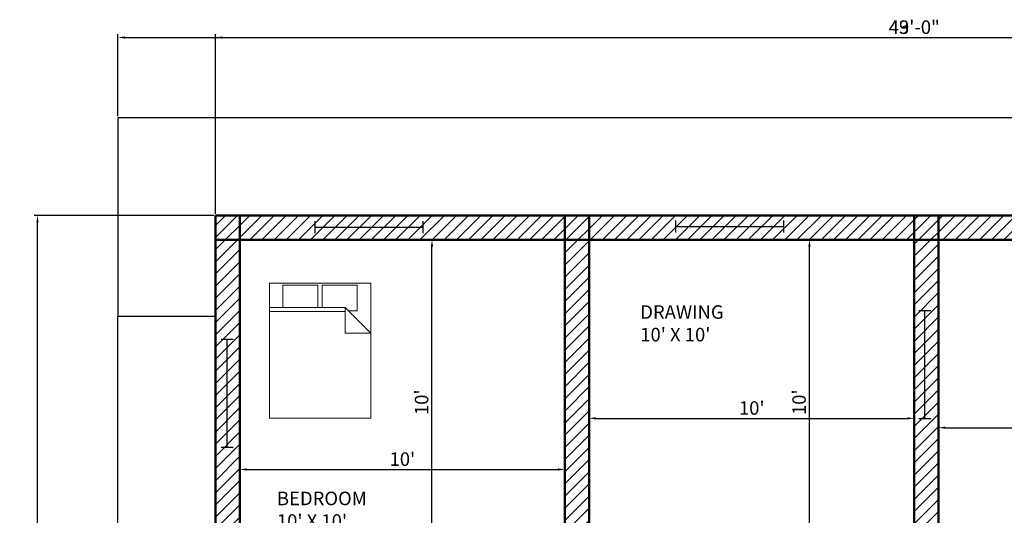
# Model space of a CAD drawing. Units: millimetres. Extents: x 2039 to 2694, y 890 to 1415.
# Tile 3 of 4: x 2039 to 2402, y 1232 to 1415. Entities that reach past the tile are written whole.
import ezdxf

# ---------------------------------------------------------------- set-up
doc = ezdxf.new("R2010")
doc.units = ezdxf.units.MM
for name, color, linetype, lineweight in [('A-ANNO-DIMS', 80, 'Continuous', 18), ('A-AREA-IDEN', 130, 'Continuous', 25), ('A-WALL-PATT', 6, 'Continuous', 13), ('C-PROP', 200, 'Continuous', 25), ('furniture', 140, 'Continuous', 18), ('walls', 200, 'Continuous', 50), ('windows', 30, 'Continuous', 25)]:
    doc.layers.add(name, color=color, linetype=linetype, lineweight=lineweight)
doc.styles.get("Standard").update_dxf_attribs({"font": 'arial.ttf'})
doc.dimstyles.new('ISO-25', dxfattribs={"dimtxt": 5, "dimasz": 2.5, "dimexe": 1.25, "dimexo": 0.625, "dimtad": 1, "dimdec": 0, "dimlunit": 3, "dimtxsty": 'Standard', "dimcen": 2.5, "dimadec": 0, "dimazin": 0, "dimtfac": 1, "dimtdec": 0, "dimtmove": 0, "dimatfit": 3, "dimfxl": 1, "dimarcsym": 0})

# ---------------------------------------------------------------- blocks, each defined once
blk = doc.blocks.new('*U4')
for p, q in [((0, 4), (0, 0)), ((36, 4), (36, 0)), ((0, 2), (36, 2))]:
    blk.add_line(p, q)
blk = doc.blocks.new('Bed - Queen')
for p, q in [((0, -80.00003), (0, 0)), ((0, 0), (59.99999, 0)), ((59.99999, 0), (59.99999, -80.00003)), ((7.99999, -1.2), (28.79998, -1.2)), ((7.99999, -14.4), (7.99999, -1.2)), ((28.79998, -1.2), (28.79998, -14.4)), ((31.19999, -1.2), (51.99999, -1.2)), ((31.19999, -14.4), (31.19999, -1.2)), ((51.99999, -1.2), (51.99999, -16.4)), ((0, -14.4), (44.8, -14.4)), ((44.8, -16.8), (0, -16.8)), ((59.99999, -29.6), (44.8, -14.4)), ((44.8, -14.4), (44.8, -29.6)), ((51.99999, -16.4), (46.79936, -16.4)), ((44.8, -29.6), (59.99999, -29.6)), ((59.99999, -80.00003), (0, -80.00003))]:
    blk.add_line(p, q)
blk = doc.blocks.new('*D8')
at = {"layer": 'A-ANNO-DIMS', "color": 0, "lineweight": -2, "transparency": 16777216}
for p, q in [((2377.91, 1235.18), (2377.91, 1265.13)), ((2617.91, 1235.18), (2617.91, 1265.13)), ((2380.41, 1263.88), (2615.41, 1263.88))]:
    blk.add_line(p, q, dxfattribs=at)
at = {"layer": 'A-ANNO-DIMS', "color": 0, "transparency": 16777216}
for points in [[(2380.41, 1264.3), (2380.41, 1263.46), (2377.91, 1263.88)], [(2615.41, 1264.3), (2615.41, 1263.46), (2617.91, 1263.88)]]:
    blk.add_solid(points, dxfattribs=at)
at = {"layer": 'Defpoints', "color": 0, "transparency": 16777216}
for p in [(2617.91, 1263.88), (2377.91, 1234.56), (2617.91, 1234.56)]:
    blk.add_point(p, dxfattribs=at)
at = {"layer": 'A-ANNO-DIMS', "color": 0, "transparency": 16777216, "insert": (2497.91, 1267.06), "char_height": 5, "attachment_point": 5}
blk.add_mtext("20'", dxfattribs=at)
blk = doc.blocks.new('*D10')
at = {"layer": 'A-ANNO-DIMS', "color": 0, "lineweight": -2, "transparency": 16777216}
for p, q in [((2119.91, 1237.17), (2119.91, 1249.7)), ((2122.41, 1248.45), (2237.41, 1248.45)), ((2239.91, 1237.17), (2239.91, 1249.7))]:
    blk.add_line(p, q, dxfattribs=at)
at = {"layer": 'A-ANNO-DIMS', "color": 0, "transparency": 16777216}
for points in [[(2122.41, 1248.87), (2122.41, 1248.03), (2119.91, 1248.45)], [(2237.41, 1248.87), (2237.41, 1248.03), (2239.91, 1248.45)]]:
    blk.add_solid(points, dxfattribs=at)
at = {"layer": 'Defpoints', "color": 0, "transparency": 16777216}
for p in [(2239.91, 1248.45), (2119.91, 1236.55), (2239.91, 1236.55)]:
    blk.add_point(p, dxfattribs=at)
at = {"layer": 'A-ANNO-DIMS', "color": 0, "transparency": 16777216, "insert": (2179.91, 1251.63), "char_height": 5, "attachment_point": 5}
blk.add_mtext("10'", dxfattribs=at)
blk = doc.blocks.new('*D11')
at = {"layer": 'A-ANNO-DIMS', "color": 0, "lineweight": -2, "transparency": 16777216}
for p, q in [((2187.65, 1333.28), (2192.09, 1333.28)), ((2190.84, 1215.78), (2190.84, 1330.78)), ((2187.65, 1213.28), (2192.09, 1213.28))]:
    blk.add_line(p, q, dxfattribs=at)
at = {"layer": 'A-ANNO-DIMS', "color": 0, "transparency": 16777216}
for points in [[(2190.42, 1330.78), (2191.26, 1330.78), (2190.84, 1333.28)], [(2190.42, 1215.78), (2191.26, 1215.78), (2190.84, 1213.28)]]:
    blk.add_solid(points, dxfattribs=at)
at = {"layer": 'Defpoints', "color": 0, "transparency": 16777216}
for p in [(2187.03, 1333.28), (2190.84, 1333.28), (2187.03, 1213.28)]:
    blk.add_point(p, dxfattribs=at)
at = {"layer": 'A-ANNO-DIMS', "color": 0, "transparency": 16777216, "insert": (2187.66, 1273.28), "char_height": 5, "attachment_point": 5, "rotation": 90}
blk.add_mtext("10'", dxfattribs=at)
blk = doc.blocks.new('*D12')
at = {"layer": 'A-ANNO-DIMS', "color": 0, "lineweight": -2, "transparency": 16777216}
for p, q in [((2248.91, 1295.38), (2248.91, 1266.07)), ((2368.91, 1295.38), (2368.91, 1266.07)), ((2251.41, 1267.32), (2366.41, 1267.32))]:
    blk.add_line(p, q, dxfattribs=at)
at = {"layer": 'A-ANNO-DIMS', "color": 0, "transparency": 16777216}
for points in [[(2251.41, 1267.74), (2251.41, 1266.91), (2248.91, 1267.32)], [(2366.41, 1267.74), (2366.41, 1266.91), (2368.91, 1267.32)]]:
    blk.add_solid(points, dxfattribs=at)
at = {"layer": 'Defpoints', "color": 0, "transparency": 16777216}
for p in [(2248.91, 1296.01), (2368.91, 1296.01), (2368.91, 1267.32)]:
    blk.add_point(p, dxfattribs=at)
at = {"layer": 'A-ANNO-DIMS', "color": 0, "transparency": 16777216, "insert": (2308.91, 1270.5), "char_height": 5, "attachment_point": 5}
blk.add_mtext("10'", dxfattribs=at)
blk = doc.blocks.new('*D13')
at = {"layer": 'A-ANNO-DIMS', "color": 0, "lineweight": -2, "transparency": 16777216}
for p, q in [((2326.26, 1333.28), (2331.46, 1333.28)), ((2330.21, 1215.78), (2330.21, 1330.78)), ((2326.26, 1213.28), (2331.46, 1213.28))]:
    blk.add_line(p, q, dxfattribs=at)
at = {"layer": 'A-ANNO-DIMS', "color": 0, "transparency": 16777216}
for points in [[(2329.79, 1330.78), (2330.63, 1330.78), (2330.21, 1333.28)], [(2329.79, 1215.78), (2330.63, 1215.78), (2330.21, 1213.28)]]:
    blk.add_solid(points, dxfattribs=at)
at = {"layer": 'Defpoints', "color": 0, "transparency": 16777216}
for p in [(2325.64, 1333.28), (2330.21, 1333.28), (2325.64, 1213.28)]:
    blk.add_point(p, dxfattribs=at)
at = {"layer": 'A-ANNO-DIMS', "color": 0, "transparency": 16777216, "insert": (2327.03, 1273.28), "char_height": 5, "attachment_point": 5, "rotation": 90}
blk.add_mtext("10'", dxfattribs=at)
blk = doc.blocks.new('*D35')
at = {"layer": 'A-ANNO-DIMS', "color": 0, "lineweight": -2, "transparency": 16777216}
for p, q in [((2110.91, 1342.9), (2110.91, 1409.23)), ((2113.41, 1407.98), (2624.41, 1407.98)), ((2626.91, 1342.9), (2626.91, 1409.23))]:
    blk.add_line(p, q, dxfattribs=at)
at = {"layer": 'A-ANNO-DIMS', "color": 0, "transparency": 16777216}
for points in [[(2113.41, 1408.39), (2113.41, 1407.56), (2110.91, 1407.98)], [(2624.41, 1408.39), (2624.41, 1407.56), (2626.91, 1407.98)]]:
    blk.add_solid(points, dxfattribs=at)
at = {"layer": 'Defpoints', "color": 0, "transparency": 16777216}
for p in [(2626.91, 1407.98), (2110.91, 1342.28), (2626.91, 1342.28)]:
    blk.add_point(p, dxfattribs=at)
at = {"layer": 'A-ANNO-DIMS', "color": 0, "transparency": 16777216, "insert": (2368.91, 1411.16), "char_height": 5, "attachment_point": 5}
blk.add_mtext('43\'-0"', dxfattribs=at)
blk = doc.blocks.new('*D36')
at = {"layer": 'A-ANNO-DIMS', "color": 0, "lineweight": -2, "transparency": 16777216}
for p, q in [((2110.28, 1342.28), (2043.96, 1342.28)), ((2045.21, 941.78), (2045.21, 1339.78)), ((2110.28, 939.28), (2043.96, 939.28))]:
    blk.add_line(p, q, dxfattribs=at)
at = {"layer": 'A-ANNO-DIMS', "color": 0, "transparency": 16777216}
for points in [[(2044.79, 1339.78), (2045.62, 1339.78), (2045.21, 1342.28)], [(2044.79, 941.78), (2045.62, 941.78), (2045.21, 939.28)]]:
    blk.add_solid(points, dxfattribs=at)
at = {"layer": 'Defpoints', "color": 0, "transparency": 16777216}
for p in [(2045.21, 1342.28), (2110.91, 1342.28), (2110.91, 939.28)]:
    blk.add_point(p, dxfattribs=at)
at = {"layer": 'A-ANNO-DIMS', "color": 0, "transparency": 16777216, "insert": (2042.03, 1140.78), "char_height": 5, "attachment_point": 5, "rotation": 90}
blk.add_mtext('33\'-7"', dxfattribs=at)
blk = doc.blocks.new('*D37')
at = {"layer": 'A-ANNO-DIMS', "color": 0, "lineweight": -2, "transparency": 16777216}
for p, q in [((2074.91, 1378.9), (2074.91, 1409.23)), ((2077.41, 1407.98), (2660.41, 1407.98)), ((2662.91, 1378.9), (2662.91, 1409.23))]:
    blk.add_line(p, q, dxfattribs=at)
at = {"layer": 'A-ANNO-DIMS', "color": 0, "transparency": 16777216}
for points in [[(2077.41, 1408.39), (2077.41, 1407.56), (2074.91, 1407.98)], [(2660.41, 1408.39), (2660.41, 1407.56), (2662.91, 1407.98)]]:
    blk.add_solid(points, dxfattribs=at)
at = {"layer": 'Defpoints', "color": 0, "transparency": 16777216}
for p in [(2662.91, 1407.98), (2074.91, 1378.28), (2662.91, 1378.28)]:
    blk.add_point(p, dxfattribs=at)
at = {"layer": 'A-ANNO-DIMS', "color": 0, "transparency": 16777216, "insert": (2368.91, 1411.15), "char_height": 5, "attachment_point": 5}
blk.add_mtext('49\'-0"', dxfattribs=at)

msp = doc.modelspace()

# ---------------------------------------------------------------- hatches: boundary and pattern name
at = {"layer": 'A-WALL-PATT'}
h = msp.add_hatch(dxfattribs=at)
h.set_pattern_fill('ANSI31', color=256)
h.paths.add_polyline_path([(2119.91, 1333.28), (2110.91, 1333.28), (2110.91, 1213.28), (2119.91, 1213.28)])
h.paths.add_polyline_path([(2119.91, 1342.28), (2110.91, 1342.28), (2110.91, 1333.28), (2119.91, 1333.28)])
h.paths.add_polyline_path([(2239.91, 1342.28), (2119.91, 1342.28), (2119.91, 1333.28), (2239.91, 1333.28)])
h.paths.add_polyline_path([(2368.91, 1342.28), (2248.91, 1342.28), (2248.91, 1333.28), (2368.91, 1333.28)])
h.paths.add_polyline_path([(2248.91, 1342.28), (2239.91, 1342.28), (2239.91, 1333.28), (2248.91, 1333.28)])
h.paths.add_polyline_path([(2248.91, 1333.28), (2239.91, 1333.28), (2239.91, 1213.28), (2248.91, 1213.28)])
h.paths.add_polyline_path([(2203.91, 1213.28), (2119.91, 1213.28), (2119.91, 1204.28), (2203.91, 1204.28)])
h.paths.add_polyline_path([(2119.91, 1204.28), (2110.91, 1204.28), (2110.91, 1156.28), (2119.91, 1156.28)])
h.paths.add_polyline_path([(2119.91, 1213.28), (2110.91, 1213.28), (2110.91, 1204.28), (2119.91, 1204.28)])
h.paths.add_polyline_path([(2212.91, 1213.28), (2203.91, 1213.28), (2203.91, 1204.28), (2212.91, 1204.28)])
h.paths.add_polyline_path([(2368.91, 1213.28), (2273.37, 1213.28, -0.081603), (2274.54, 1206.12), (2274.54, 1204.28), (2368.91, 1204.28)])
h.paths.add_polyline_path([(2377.91, 1333.28), (2368.91, 1333.28), (2368.91, 1213.28), (2377.91, 1213.28)])
h.paths.add_polyline_path([(2617.91, 1342.28), (2377.91, 1342.28), (2377.91, 1333.28), (2617.91, 1333.28)])
h.paths.add_polyline_path([(2377.91, 1342.28), (2368.91, 1342.28), (2368.91, 1333.28), (2377.91, 1333.28)])
h.paths.add_polyline_path([(2626.91, 1333.28), (2617.91, 1333.28), (2617.91, 948.28), (2626.91, 948.28)])
h.paths.add_polyline_path([(2377.91, 1204.28), (2368.91, 1204.28), (2368.91, 1156.28), (2377.91, 1156.28)])
h.paths.add_polyline_path([(2377.91, 1156.28), (2368.91, 1156.28), (2368.91, 1147.28), (2377.91, 1147.28)])
h.paths.add_polyline_path([(2377.91, 1213.28), (2368.91, 1213.28), (2368.91, 1204.28), (2377.91, 1204.28)])
h.paths.add_polyline_path([(2368.91, 1156.28), (2360.56, 1156.28), (2360.56, 1148.39), (2360.56, 1147.28), (2368.91, 1147.28)])
h.paths.add_polyline_path([(2399.91, 1156.28), (2377.91, 1156.28), (2377.91, 1147.28), (2399.91, 1147.28)])
h.paths.add_polyline_path([(2408.91, 1156.28), (2399.91, 1156.28), (2399.91, 1147.28), (2408.91, 1147.28)])
h.paths.add_polyline_path([(2339.63, 1156.28), (2327.91, 1156.28), (2327.91, 1147.28), (2338.19, 1147.28), (2338.19, 1148.39, -0.090365)])
h.paths.add_polyline_path([(2327.91, 1156.28), (2318.91, 1156.28), (2318.91, 1147.28), (2327.91, 1147.28)])
h.paths.add_polyline_path([(2327.91, 1147.28), (2318.91, 1147.28), (2318.91, 1041.28), (2327.91, 1041.28)])
h.paths.add_polyline_path([(2408.91, 1109.51), (2399.91, 1109.51), (2399.91, 948.28), (2408.91, 948.28)])
h.paths.add_polyline_path([(2272.91, 1080.28), (2263.91, 1080.28), (2263.91, 1041.28), (2272.91, 1041.28)])
h.paths.add_polyline_path([(2272.91, 1089.28), (2263.91, 1089.28), (2263.91, 1080.28), (2272.91, 1080.28)])
h.paths.add_polyline_path([(2263.91, 1089.28), (2252.09, 1089.28), (2252.48, 1080.28), (2263.91, 1080.28)])
h.paths.add_polyline_path([(2229.75, 1088.3), (2229.7, 1089.28), (2212.91, 1089.28), (2212.91, 1080.28), (2231.62, 1080.28, -0.092884)])
h.paths.add_polyline_path([(2212.91, 1124.18), (2211.56, 1124.21, -0.10492), (2203.91, 1126.01), (2203.91, 1089.28), (2212.91, 1089.28)])
h.paths.add_polyline_path([(2212.91, 1089.28), (2203.91, 1089.28), (2203.91, 1080.28), (2212.91, 1080.28)])
h.paths.add_polyline_path([(2203.91, 1089.28), (2119.91, 1089.28), (2119.91, 1080.28), (2203.91, 1080.28)])
h.paths.add_polyline_path([(2119.91, 1147.28), (2110.91, 1147.28), (2110.91, 1089.28), (2119.91, 1089.28)])
h.paths.add_polyline_path([(2119.91, 1156.28), (2110.91, 1156.28), (2110.91, 1147.28), (2119.91, 1147.28)])
h.paths.add_polyline_path([(2203.91, 1156.28), (2119.91, 1156.28), (2119.91, 1147.28), (2136.91, 1147.28), (2203.91, 1147.28)])
h.paths.add_polyline_path([(2119.91, 1080.28), (2110.91, 1080.28), (2110.91, 948.28), (2119.91, 948.28)])
h.paths.add_polyline_path([(2119.91, 1089.28), (2110.91, 1089.28), (2110.91, 1080.28), (2119.91, 1080.28)])
h.paths.add_polyline_path([(2119.91, 948.28), (2110.91, 948.28), (2110.91, 939.28), (2119.91, 939.28)])
h.paths.add_polyline_path([(2263.91, 948.28), (2119.91, 948.28), (2119.91, 939.28), (2263.91, 939.28)])
h.paths.add_polyline_path([(2318.91, 948.28), (2272.91, 948.28), (2272.91, 939.28), (2318.91, 939.28)])
h.paths.add_polyline_path([(2272.91, 948.28), (2263.91, 948.28), (2263.91, 939.28), (2272.91, 939.28)])
h.paths.add_polyline_path([(2272.91, 1041.28), (2263.91, 1041.28), (2263.91, 1032.28), (2272.91, 1032.28)])
h.paths.add_polyline_path([(2327.91, 1032.28), (2318.91, 1032.28), (2318.91, 948.28), (2327.91, 948.28)])
h.paths.add_polyline_path([(2399.91, 948.28), (2327.91, 948.28), (2327.91, 939.28), (2399.91, 939.28)])
h.paths.add_polyline_path([(2327.91, 948.28), (2318.91, 948.28), (2318.91, 939.28), (2327.91, 939.28)])
h.paths.add_polyline_path([(2408.91, 948.28), (2399.91, 948.28), (2399.91, 939.28), (2408.91, 939.28)])
h.paths.add_polyline_path([(2617.91, 948.28), (2408.91, 948.28), (2408.91, 939.28), (2617.91, 939.28)])
h.paths.add_polyline_path([(2626.91, 948.28), (2617.91, 948.28), (2617.91, 939.28), (2626.91, 939.28)])
h.paths.add_polyline_path([(2132.32, 1149.06), (2159.44, 1149.06), (2159.44, 1167.69), (2132.32, 1167.69)], flags=9)

# ---------------------------------------------------------------- linework, layer by layer
at = {"layer": 'C-PROP'}
for p, q in [((2662.91, 1378.28), (2074.91, 1378.28)), ((2074.91, 1378.28), (2074.91, 1304.98)), ((2110.91, 1304.98), (2074.91, 1304.98)), ((2074.91, 939.28), (2074.91, 1304.98))]:
    msp.add_line(p, q, dxfattribs=at)
at = {"layer": 'walls'}
for p, q in [((2110.91, 1342.28), (2110.91, 939.28)), ((2110.91, 1342.28), (2626.91, 1342.28)), ((2119.91, 1342.28), (2119.91, 939.28)), ((2239.91, 1342.28), (2239.91, 1204.28)), ((2248.91, 1342.28), (2248.91, 1204.28)), ((2368.91, 1342.28), (2368.91, 1147.28)), ((2377.91, 1342.28), (2377.91, 1147.28)), ((2110.91, 1333.28), (2626.91, 1333.28))]:
    msp.add_line(p, q, dxfattribs=at)

# ---------------------------------------------------------------- block references
at = {"layer": 'furniture', "xscale": 0.6236252200436019, "yscale": 0.6236252200436019, "zscale": 0.6236252200436019}
msp.add_blockref('Bed - Queen', (2130.79, 1317.31), dxfattribs=at)
at = {"layer": 'windows', "xscale": 1.108036427899419, "yscale": 1.108036427899419, "zscale": 1.108036427899419}
for p in [(2147.6, 1335.66), (2280.7, 1335.93)]:
    msp.add_blockref('*U4', p, dxfattribs=at)
at = {"layer": 'windows', "xscale": 1.108036427899419, "yscale": 1.108036427899419, "zscale": 1.108036427899419, "rotation": 90}
for p in [(2375.01, 1267.32), (2117.4, 1256.73)]:
    msp.add_blockref('*U4', p, dxfattribs=at)

# ---------------------------------------------------------------- texts
at = {"layer": 'A-AREA-IDEN', "char_height": 5, "attachment_point": 1}
for s, width, insert in [("DRAWING\\P10' X 10'", 46.6908, (2267.74, 1309.09)), ("BEDROOM\\P10' X 10'", 49.8516, (2133.59, 1240.25))]:
    msp.add_mtext_dynamic_manual_height_columns(s, width=width, gutter_width=12.5, heights=[0], dxfattribs=dict(at, insert=insert))

# ---------------------------------------------------------------- dimensions: what is measured, and where the dimension line sits
at = {"layer": 'A-ANNO-DIMS'}
for base, p1, p2, override, picture, middle in [((2662.91, 1407.98), (2074.91, 1378.28), (2662.91, 1378.28), {"dimdec": 1, "dimlfac": 1, "dimrnd": 0, "dimzin": 1, "dimdsep": 46, "dimlunit": 4, "dimfrac": 2}, '*D37', (2368.91, 1411.15)), ((2626.91, 1407.98), (2110.91, 1342.28), (2626.91, 1342.28), {"dimdec": 1, "dimlfac": 1, "dimrnd": 0, "dimzin": 1, "dimdsep": 46, "dimlunit": 4, "dimfrac": 2}, '*D35', (2368.91, 1411.16)), ((2368.91, 1267.32), (2248.91, 1296.01), (2368.91, 1296.01), {"dimclrd": 0, "dimclre": 0, "dimclrt": 0}, '*D12', (2308.91, 1270.5)), ((2617.91, 1263.88), (2377.91, 1234.56), (2617.91, 1234.56), {"dimclrd": 0, "dimclre": 0, "dimclrt": 0}, '*D8', (2497.91, 1267.06)), ((2239.91, 1248.45), (2119.91, 1236.55), (2239.91, 1236.55), {"dimclrd": 0, "dimclre": 0, "dimclrt": 0}, '*D10', (2179.91, 1251.63))]:
    dim = msp.add_linear_dim(base=base, p1=p1, p2=p2, dimstyle='ISO-25', override=override, dxfattribs=at)
    dim.commit()
    dim.dimension.update_dxf_attribs({"geometry": picture, "text_midpoint": middle})
for base, p1, p2, override, picture, middle in [((2045.21, 1342.28), (2110.91, 939.28), (2110.91, 1342.28), {"dimdec": 1, "dimlfac": 1, "dimrnd": 0, "dimzin": 1, "dimdsep": 46, "dimlunit": 4, "dimfrac": 2}, '*D36', (2042.03, 1140.78)), ((2190.84, 1333.28), (2187.03, 1213.28), (2187.03, 1333.28), {"dimclrd": 0, "dimclre": 0, "dimclrt": 0}, '*D11', (2187.66, 1273.28)), ((2330.21, 1333.28), (2325.64, 1213.28), (2325.64, 1333.28), {"dimclrd": 0, "dimclre": 0, "dimclrt": 0}, '*D13', (2327.03, 1273.28))]:
    dim = msp.add_linear_dim(base=base, p1=p1, p2=p2, angle=90, dimstyle='ISO-25', override=override, dxfattribs=at)
    dim.commit()
    dim.dimension.update_dxf_attribs({"geometry": picture, "text_midpoint": middle})

doc.saveas('drawing.dxf')
